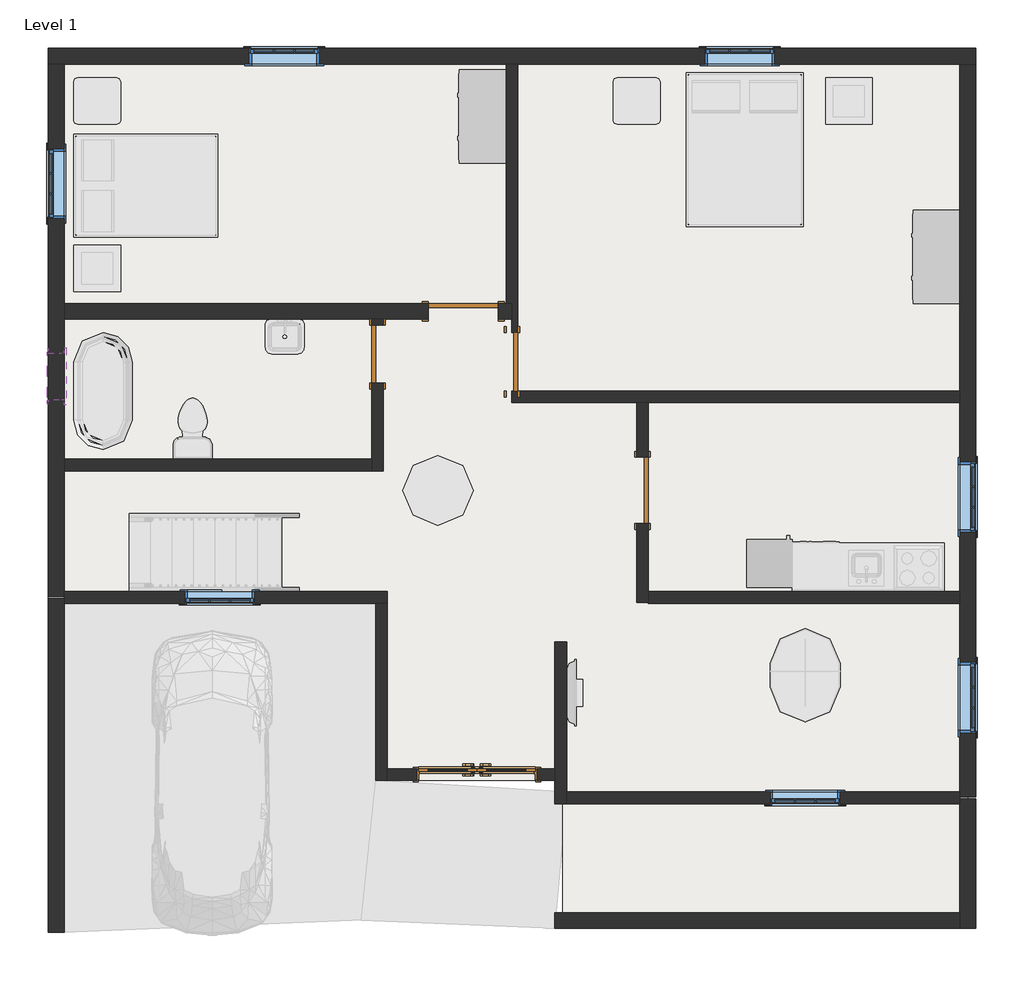
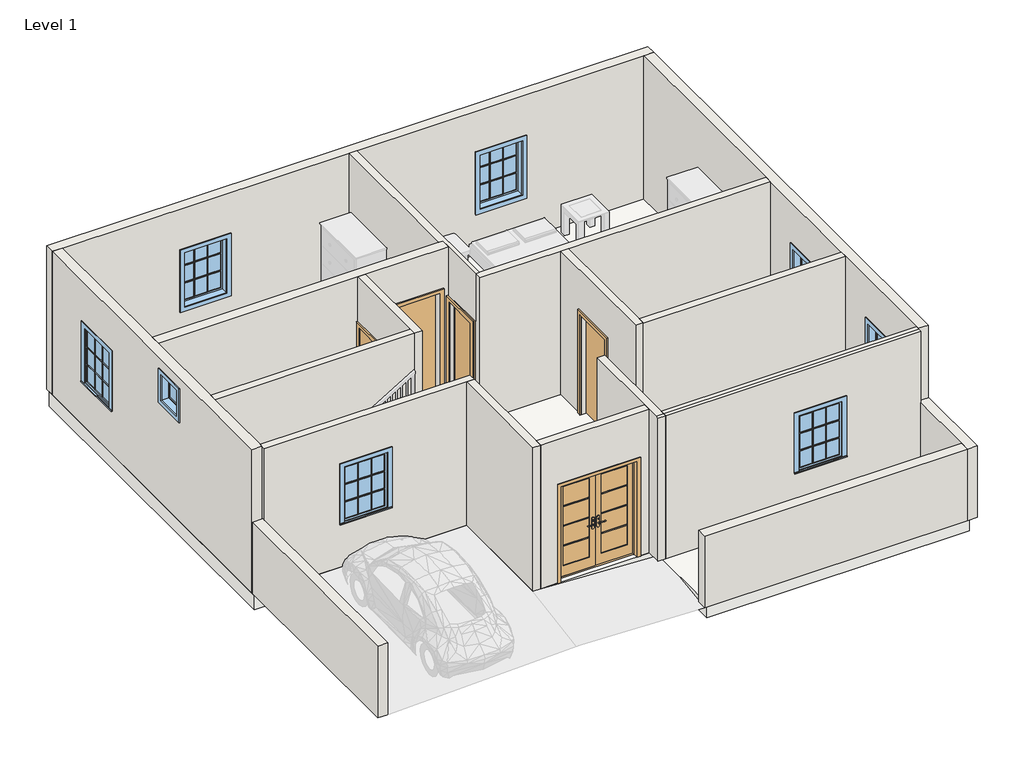
# One storey, part 1 of 2: 18 walls, 8 windows, 5 doors, 1 slab.
"""IFC4 building model written with IfcOpenShell, lengths in millimetres."""

from ifc_helpers import new_model, si_unit, frame, origin, origin_with_axes, place, context, project, spatial, polyline, outline, extrude, faceted_brep, transform, mapped, element, save
from components import door_94998e6c, door_059fdd7e, door_99d96fc5, door_54dd4da4, window_29c06734, window_5c190c7e, window_e41d21a6

model = new_model("IFC4")

# Units and contexts
model_context = context("Model", 3, world=origin())
ifc_project = project(units=[si_unit("LENGTHUNIT", "METRE", prefix="MILLI")], contexts=[model_context])

# Site, building, storey
site = spatial("IfcSite", under=ifc_project)
building = spatial("IfcBuilding", under=site)
storey = spatial("IfcBuildingStorey", under=building, Name="Level 1", Elevation=0.0)

# Doors
placement = place(None, origin())
door_shape = door_94998e6c(model_context)
element("IfcDoor", 1, ObjectType="Door-Exterior-Double-Full Glass-Wood_Clad : 60\" x 80\"", at=placement, inside=storey, context=model_context, shape_type="MappedRepresentation", body=[
    mapped(door_shape, transform((-8502.4576657, 4160.7479822, 0.0), x_axis=(1.0, 0.0, 0.0), y_axis=(0.0, 1.0, 0.0), z_axis=(0.0, 0.0, 1.0))),
])
door_2_shape = door_059fdd7e(model_context)
element("IfcDoor", 2, ObjectType="Single-Flush : 30\" x 80\"", at=placement, inside=storey, context=model_context, shape_type="MappedRepresentation", body=[
    mapped(door_2_shape, transform((-9797.8576657, 9643.9729822, 0.0), x_axis=(0.0, 1.0, 0.0), y_axis=(-1.0, 0.0, 0.0), z_axis=(0.0, 0.0, 1.0))),
])
element("IfcDoor", 3, ObjectType="Single-Flush : 30\" x 80\"", at=placement, inside=storey, context=model_context, shape_type="MappedRepresentation", body=[
    mapped(door_2_shape, transform((-8045.2576657, 9542.3729822, 0.0), x_axis=(0.0, -1.0, 0.0), y_axis=(1.0, 0.0, 0.0), z_axis=(0.0, 0.0, 1.0))),
])
door_3_shape = door_99d96fc5(model_context)
element("IfcDoor", 4, ObjectType="Single-Flush : 34\" x 84\"", at=placement, inside=storey, context=model_context, shape_type="MappedRepresentation", body=[
    mapped(door_3_shape, transform((-6343.4576657, 7865.9729822, 0.0), x_axis=(0.0, 1.0, 0.0), y_axis=(-1.0, 0.0, 0.0), z_axis=(0.0, 0.0, 1.0))),
])
door_4_shape = door_54dd4da4(model_context)
element("IfcDoor", 5, ObjectType="Single-Flush : 36\" x 84\"", at=placement, inside=storey, context=model_context, shape_type="MappedRepresentation", body=[
    mapped(door_4_shape, transform((-8680.2576657, 10202.7729822, 0.0), x_axis=(1.0, 0.0, 0.0), y_axis=(0.0, 1.0, 0.0), z_axis=(0.0, 0.0, 1.0))),
])

# Slab
element("IfcSlab", 6, ObjectType="Generic - 12\"", at=placement, inside=storey, context=model_context, shape_type="SweptSolid", body=[
    extrude(outline(polyline([(-2101.6576657, 13530.1729822), (-2101.6576657, 2252.5729822), (-7384.8576657, 2252.5729822), (-7384.8576657, 4081.3729822), (-9823.2576657, 4081.3729822), (-9823.2576657, 6392.7729822), (-14090.4576657, 6392.7729822), (-14090.4576657, 13530.1729822), (-2101.6576657, 13530.1729822)])), frame((0.0, 0.0, -304.8), z_axis=(0.0, 0.0, 1.0), x_axis=(1.0, 0.0, 0.0)), (0.0, 0.0, 1.0), 304.8),
])

# Walls
element("IfcWall", 7, ObjectType="Generic - 5'", at=placement, inside=storey, context=model_context, shape_type="SweptSolid", body=[
    extrude(outline(polyline([(-7486.4576657, 2354.1729822), (-2203.2576657, 2354.1729822), (-2203.2576657, 2150.9729822), (-7486.4576657, 2150.9729822), (-7486.4576657, 2354.1729822)])), origin_with_axes(), (0.0, 0.0, 1.0), 1524.0),
])
element("IfcWall", 8, ObjectType="Generic - 5'", at=placement, inside=storey, context=model_context, shape_type="SweptSolid", body=[
    extrude(outline(polyline([(-13887.2576657, 6456.2729822), (-13887.2576657, 2100.1729822), (-14090.4576657, 2100.1729822), (-14090.4576657, 6456.2729822), (-13887.2576657, 6456.2729822)])), origin_with_axes(), (0.0, 0.0, 1.0), 1524.0),
])
element("IfcWall", 9, ObjectType="Generic - 5'", at=placement, inside=storey, context=model_context, shape_type="Brep", body=[
    faceted_brep([(-2203.2576657, 3840.0729822, 0.0), (-2203.2576657, 3776.5729822, 0.0), (-2203.2576657, 2354.1729822, 0.0), (-2203.2576657, 2150.9729822, 0.0), (-2203.2576657, 2150.9729822, 1524.0), (-2203.2576657, 2354.1729822, 1524.0), (-2203.2576657, 3840.0729822, 1524.0), (-2000.0576657, 3840.0729822, 0.0), (-2000.0576657, 3840.0729822, 1524.0), (-2000.0576657, 2150.9729822, 1524.0), (-2000.0576657, 2150.9729822, 0.0)], [[[0, 1, 2, 3, 4, 5, 6]], [[7, 8, 9, 10]], [[3, 2, 1, 0, 7, 10]], [[6, 5, 4, 9, 8]], [[0, 6, 8, 7]], [[4, 3, 10, 9]]]),
])
element("IfcWall", 10, ObjectType="Generic - 8\"", at=placement, inside=storey, context=model_context, shape_type="Brep", body=[
    faceted_brep([(-14090.4576657, 13428.5729822, 0.0), (-13887.2576657, 13428.5729822, 0.0), (-8121.4576657, 13428.5729822, 0.0), (-7969.0576657, 13428.5729822, 0.0), (-2203.2576657, 13428.5729822, 0.0), (-2000.0576657, 13428.5729822, 0.0), (-2000.0576657, 13428.5729822, 3048.0), (-2203.2576657, 13428.5729822, 3048.0), (-7969.0576657, 13428.5729822, 3048.0), (-8121.4576657, 13428.5729822, 3048.0), (-13887.2576657, 13428.5729822, 3048.0), (-14090.4576657, 13428.5729822, 3048.0), (-10559.8576657, 13428.5729822, 2133.6), (-10559.8576657, 13428.5729822, 914.4), (-11474.2576657, 13428.5729822, 914.4), (-11474.2576657, 13428.5729822, 2133.6), (-4616.2576657, 13428.5729822, 2133.6), (-4616.2576657, 13428.5729822, 914.4), (-5530.6576657, 13428.5729822, 914.4), (-5530.6576657, 13428.5729822, 2133.6), (-14090.4576657, 13631.7729822, 0.0), (-14090.4576657, 13631.7729822, 3048.0), (-2000.0576657, 13631.7729822, 3048.0), (-2000.0576657, 13631.7729822, 0.0), (-10559.8576657, 13631.7729822, 2133.6), (-11474.2576657, 13631.7729822, 2133.6), (-11474.2576657, 13631.7729822, 914.4), (-10559.8576657, 13631.7729822, 914.4), (-4616.2576657, 13631.7729822, 2133.6), (-5530.6576657, 13631.7729822, 2133.6), (-5530.6576657, 13631.7729822, 914.4), (-4616.2576657, 13631.7729822, 914.4)], [[[0, 1, 2, 3, 4, 5, 6, 7, 8, 9, 10, 11], [12, 13, 14, 15], [16, 17, 18, 19]], [[20, 21, 22, 23], [24, 25, 26, 27], [28, 29, 30, 31]], [[5, 4, 3, 2, 1, 0, 20, 23]], [[6, 5, 23, 22]], [[0, 11, 21, 20]], [[13, 12, 24, 27]], [[14, 13, 27, 26]], [[15, 14, 26, 25]], [[12, 15, 25, 24]], [[17, 16, 28, 31]], [[18, 17, 31, 30]], [[19, 18, 30, 29]], [[16, 19, 29, 28]], [[11, 10, 9, 8, 7, 6, 22, 21]]]),
])
element("IfcWall", 11, ObjectType="Generic - 8\"", at=placement, inside=storey, context=model_context, shape_type="Brep", body=[
    faceted_brep([(-2203.2576657, 13428.5729822, 0.0), (-2203.2576657, 9161.3729822, 0.0), (-2203.2576657, 9008.9729822, 0.0), (-2203.2576657, 6545.1729822, 0.0), (-2203.2576657, 6392.7729822, 0.0), (-2203.2576657, 3865.4729822, 0.0), (-2203.2576657, 3865.4729822, 3048.0), (-2203.2576657, 6392.7729822, 3048.0), (-2203.2576657, 6545.1729822, 3048.0), (-2203.2576657, 9008.9729822, 3048.0), (-2203.2576657, 9161.3729822, 3048.0), (-2203.2576657, 13428.5729822, 3048.0), (-2203.2576657, 7319.8729822, 2133.6), (-2203.2576657, 7319.8729822, 914.4), (-2203.2576657, 8234.2729822, 914.4), (-2203.2576657, 8234.2729822, 2133.6), (-2203.2576657, 4703.6729822, 2133.6), (-2203.2576657, 4703.6729822, 914.4), (-2203.2576657, 5618.0729822, 914.4), (-2203.2576657, 5618.0729822, 2133.6), (-2000.0576657, 13428.5729822, 0.0), (-2000.0576657, 13428.5729822, 3048.0), (-2000.0576657, 3865.4729822, 3048.0), (-2000.0576657, 3865.4729822, 0.0), (-2000.0576657, 7319.8729822, 2133.6), (-2000.0576657, 8234.2729822, 2133.6), (-2000.0576657, 8234.2729822, 914.4), (-2000.0576657, 7319.8729822, 914.4), (-2000.0576657, 4703.6729822, 2133.6), (-2000.0576657, 5618.0729822, 2133.6), (-2000.0576657, 5618.0729822, 914.4), (-2000.0576657, 4703.6729822, 914.4)], [[[0, 1, 2, 3, 4, 5, 6, 7, 8, 9, 10, 11], [12, 13, 14, 15], [16, 17, 18, 19]], [[20, 21, 22, 23], [24, 25, 26, 27], [28, 29, 30, 31]], [[5, 4, 3, 2, 1, 0, 20, 23]], [[6, 5, 23, 22]], [[0, 11, 21, 20]], [[13, 12, 24, 27]], [[14, 13, 27, 26]], [[15, 14, 26, 25]], [[12, 15, 25, 24]], [[17, 16, 28, 31]], [[18, 17, 31, 30]], [[19, 18, 30, 29]], [[16, 19, 29, 28]], [[11, 10, 9, 8, 7, 6, 22, 21]]]),
])
element("IfcWall", 12, ObjectType="Generic - 8\"", at=placement, inside=storey, context=model_context, shape_type="Brep", body=[
    faceted_brep([(-8045.2576657, 10304.3729822, 0.0), (-8121.4576657, 10304.3729822, 0.0), (-8223.0576657, 10304.3729822, 0.0), (-8223.0576657, 10304.3729822, 2133.6), (-9137.4576657, 10304.3729822, 2133.6), (-9137.4576657, 10304.3729822, 0.0), (-13887.2576657, 10304.3729822, 0.0), (-13887.2576657, 10304.3729822, 3048.0), (-8121.4576657, 10304.3729822, 3048.0), (-8045.2576657, 10304.3729822, 3048.0), (-8223.0576657, 10101.1729822, 2133.6), (-8223.0576657, 10101.1729822, 0.0), (-8045.2576657, 10101.1729822, 0.0), (-8045.2576657, 10101.1729822, 3048.0), (-9721.6576657, 10101.1729822, 3048.0), (-9874.0576657, 10101.1729822, 3048.0), (-13887.2576657, 10101.1729822, 3048.0), (-13887.2576657, 10101.1729822, 0.0), (-9874.0576657, 10101.1729822, 0.0), (-9721.6576657, 10101.1729822, 0.0), (-9137.4576657, 10101.1729822, 0.0), (-9137.4576657, 10101.1729822, 2133.6)], [[[0, 1, 2, 3, 4, 5, 6, 7, 8, 9]], [[10, 11, 12, 13, 14, 15, 16, 17, 18, 19, 20, 21]], [[12, 11, 2, 1, 0]], [[20, 19, 18, 17, 6, 5]], [[0, 9, 13, 12]], [[7, 6, 17, 16]], [[3, 2, 11, 10]], [[4, 3, 10, 21]], [[5, 4, 21, 20]], [[9, 8, 7, 16, 15, 14, 13]]]),
])
element("IfcWall", 13, ObjectType="Generic - 8\"", at=placement, inside=storey, context=model_context, shape_type="Brep", body=[
    faceted_brep([(-13887.2576657, 6481.6729822, 0.0), (-13887.2576657, 6545.1729822, 0.0), (-13887.2576657, 8119.9729822, 0.0), (-13887.2576657, 8272.3729822, 0.0), (-13887.2576657, 10101.1729822, 0.0), (-13887.2576657, 10304.3729822, 0.0), (-13887.2576657, 13428.5729822, 0.0), (-13887.2576657, 13428.5729822, 3048.0), (-13887.2576657, 10304.3729822, 3048.0), (-13887.2576657, 10101.1729822, 3048.0), (-13887.2576657, 8272.3729822, 3048.0), (-13887.2576657, 8119.9729822, 3048.0), (-13887.2576657, 6545.1729822, 3048.0), (-13887.2576657, 6481.6729822, 3048.0), (-13887.2576657, 12323.6729822, 2133.6), (-13887.2576657, 12323.6729822, 914.4), (-13887.2576657, 11409.2729822, 914.4), (-13887.2576657, 11409.2729822, 2133.6), (-13887.2576657, 9047.0729822, 2768.6), (-13887.2576657, 9656.6729822, 2768.6), (-13887.2576657, 9656.6729822, 2159.0), (-13887.2576657, 9047.0729822, 2159.0), (-14090.4576657, 6481.6729822, 0.0), (-14090.4576657, 6481.6729822, 3048.0), (-14090.4576657, 13428.5729822, 3048.0), (-14090.4576657, 13428.5729822, 0.0), (-14090.4576657, 12323.6729822, 2133.6), (-14090.4576657, 11409.2729822, 2133.6), (-14090.4576657, 11409.2729822, 914.4), (-14090.4576657, 12323.6729822, 914.4), (-14090.4576657, 9047.0729822, 2768.6), (-14090.4576657, 9047.0729822, 2159.0), (-14090.4576657, 9656.6729822, 2159.0), (-14090.4576657, 9656.6729822, 2768.6)], [[[0, 1, 2, 3, 4, 5, 6, 7, 8, 9, 10, 11, 12, 13], [14, 15, 16, 17], [18, 19, 20, 21]], [[22, 23, 24, 25], [26, 27, 28, 29], [30, 31, 32, 33]], [[6, 5, 4, 3, 2, 1, 0, 22, 25]], [[0, 13, 23, 22]], [[7, 6, 25, 24]], [[14, 17, 27, 26]], [[17, 16, 28, 27]], [[16, 15, 29, 28]], [[15, 14, 26, 29]], [[30, 33, 19, 18]], [[33, 32, 20, 19]], [[32, 31, 21, 20]], [[31, 30, 18, 21]], [[13, 12, 11, 10, 9, 8, 7, 24, 23]]]),
])
element("IfcWall", 14, ObjectType="INNER 6\"", at=placement, inside=storey, context=model_context, shape_type="Brep", body=[
    faceted_brep([(-8121.4576657, 13428.5729822, 0.0), (-8121.4576657, 10304.3729822, 0.0), (-8121.4576657, 10304.3729822, 3048.0), (-8121.4576657, 13428.5729822, 3048.0), (-7969.0576657, 13428.5729822, 0.0), (-7969.0576657, 13428.5729822, 3048.0), (-7969.0576657, 9161.3729822, 3048.0), (-7969.0576657, 9161.3729822, 2032.0), (-7969.0576657, 9923.3729822, 2032.0), (-7969.0576657, 9923.3729822, 0.0), (-8045.2576657, 9923.3729822, 0.0), (-8045.2576657, 10101.1729822, 0.0), (-8045.2576657, 10304.3729822, 0.0), (-8045.2576657, 10304.3729822, 3048.0), (-8045.2576657, 9923.3729822, 2032.0), (-8045.2576657, 9161.3729822, 2032.0), (-8045.2576657, 9161.3729822, 3048.0), (-8045.2576657, 10101.1729822, 3048.0)], [[[0, 1, 2, 3]], [[4, 5, 6, 7, 8, 9]], [[1, 0, 4, 9, 10, 11, 12]], [[0, 3, 5, 4]], [[2, 1, 12, 13]], [[13, 12, 11, 10, 14, 15, 16, 17]], [[6, 16, 15, 7]], [[14, 8, 7, 15]], [[8, 14, 10, 9]], [[3, 2, 13, 17, 16, 6, 5]]]),
])
element("IfcWall", 15, ObjectType="INNER 6\"", at=placement, inside=storey, context=model_context, shape_type="Brep", body=[
    faceted_brep([(-2203.2576657, 9161.3729822, 0.0), (-8045.2576657, 9161.3729822, 0.0), (-8045.2576657, 9161.3729822, 2032.0), (-8045.2576657, 9161.3729822, 3048.0), (-7969.0576657, 9161.3729822, 3048.0), (-2203.2576657, 9161.3729822, 3048.0), (-2203.2576657, 9008.9729822, 0.0), (-2203.2576657, 9008.9729822, 3048.0), (-6267.2576657, 9008.9729822, 3048.0), (-6419.6576657, 9008.9729822, 3048.0), (-8045.2576657, 9008.9729822, 3048.0), (-8045.2576657, 9008.9729822, 0.0), (-6419.6576657, 9008.9729822, 0.0), (-6267.2576657, 9008.9729822, 0.0)], [[[0, 1, 2, 3, 4, 5]], [[6, 7, 8, 9, 10, 11, 12, 13]], [[1, 0, 6, 13, 12, 11]], [[3, 2, 1, 11, 10]], [[0, 5, 7, 6]], [[5, 4, 3, 10, 9, 8, 7]]]),
])
element("IfcWall", 16, ObjectType="INNER 6\"", at=placement, inside=storey, context=model_context, shape_type="Brep", body=[
    faceted_brep([(-9874.0576657, 10101.1729822, 0.0), (-9874.0576657, 10024.9729822, 0.0), (-9874.0576657, 10024.9729822, 2032.0), (-9874.0576657, 9262.9729822, 2032.0), (-9874.0576657, 9262.9729822, 0.0), (-9874.0576657, 8272.3729822, 0.0), (-9874.0576657, 8119.9729822, 0.0), (-9874.0576657, 8119.9729822, 3048.0), (-9874.0576657, 8272.3729822, 3048.0), (-9874.0576657, 10101.1729822, 3048.0), (-9721.6576657, 10024.9729822, 2032.0), (-9721.6576657, 10024.9729822, 0.0), (-9721.6576657, 10101.1729822, 0.0), (-9721.6576657, 10101.1729822, 3048.0), (-9721.6576657, 8119.9729822, 3048.0), (-9721.6576657, 8119.9729822, 0.0), (-9721.6576657, 9262.9729822, 0.0), (-9721.6576657, 9262.9729822, 2032.0)], [[[0, 1, 2, 3, 4, 5, 6, 7, 8, 9]], [[10, 11, 12, 13, 14, 15, 16, 17]], [[16, 15, 6, 5, 4]], [[12, 11, 1, 0]], [[0, 9, 13, 12]], [[7, 6, 15, 14]], [[2, 1, 11, 10]], [[3, 2, 10, 17]], [[4, 3, 17, 16]], [[9, 8, 7, 14, 13]]]),
])
element("IfcWall", 17, ObjectType="INNER 6\"", at=placement, inside=storey, context=model_context, shape_type="SweptSolid", body=[
    extrude(outline(polyline([(-13887.2576657, 8272.3729822), (-9874.0576657, 8272.3729822), (-9874.0576657, 8119.9729822), (-13887.2576657, 8119.9729822), (-13887.2576657, 8272.3729822)])), origin_with_axes(), (0.0, 0.0, 1.0), 3048.0),
])
element("IfcWall", 18, ObjectType="INNER 6\"", at=placement, inside=storey, context=model_context, shape_type="Brep", body=[
    faceted_brep([(-13887.2576657, 6392.7729822, 0.0), (-9823.2576657, 6392.7729822, 0.0), (-9670.8576657, 6392.7729822, 0.0), (-9670.8576657, 6392.7729822, 3048.0), (-9823.2576657, 6392.7729822, 3048.0), (-13887.2576657, 6392.7729822, 3048.0), (-12312.4576657, 6392.7729822, 2133.6), (-11398.0576657, 6392.7729822, 2133.6), (-11398.0576657, 6392.7729822, 914.4), (-12312.4576657, 6392.7729822, 914.4), (-13887.2576657, 6545.1729822, 0.0), (-13887.2576657, 6545.1729822, 3048.0), (-9670.8576657, 6545.1729822, 3048.0), (-9670.8576657, 6545.1729822, 0.0), (-12312.4576657, 6545.1729822, 2133.6), (-12312.4576657, 6545.1729822, 914.4), (-11398.0576657, 6545.1729822, 914.4), (-11398.0576657, 6545.1729822, 2133.6), (-13887.2576657, 6481.6729822, 0.0), (-13887.2576657, 6481.6729822, 3048.0)], [[[0, 1, 2, 3, 4, 5], [6, 7, 8, 9]], [[10, 11, 12, 13], [14, 15, 16, 17]], [[2, 1, 0, 18, 10, 13]], [[0, 5, 19, 11, 10, 18]], [[3, 2, 13, 12]], [[15, 14, 6, 9]], [[16, 15, 9, 8]], [[17, 16, 8, 7]], [[14, 17, 7, 6]], [[5, 4, 3, 12, 11, 19]]]),
])
element("IfcWall", 19, ObjectType="INNER 6\"", at=placement, inside=storey, context=model_context, shape_type="Brep", body=[
    faceted_brep([(-6419.6576657, 9008.9729822, 0.0), (-6419.6576657, 8297.7729822, 0.0), (-6419.6576657, 8297.7729822, 2133.6), (-6419.6576657, 7434.1729822, 2133.6), (-6419.6576657, 7434.1729822, 0.0), (-6419.6576657, 6405.4729822, 0.0), (-6419.6576657, 6405.4729822, 3048.0), (-6419.6576657, 9008.9729822, 3048.0), (-6267.2576657, 8297.7729822, 2133.6), (-6267.2576657, 8297.7729822, 0.0), (-6267.2576657, 9008.9729822, 0.0), (-6267.2576657, 9008.9729822, 3048.0), (-6267.2576657, 6545.1729822, 3048.0), (-6267.2576657, 6405.4729822, 3048.0), (-6267.2576657, 6405.4729822, 0.0), (-6267.2576657, 6545.1729822, 0.0), (-6267.2576657, 7434.1729822, 0.0), (-6267.2576657, 7434.1729822, 2133.6)], [[[0, 1, 2, 3, 4, 5, 6, 7]], [[8, 9, 10, 11, 12, 13, 14, 15, 16, 17]], [[10, 9, 1, 0]], [[16, 15, 14, 5, 4]], [[6, 5, 14, 13]], [[0, 7, 11, 10]], [[2, 1, 9, 8]], [[3, 2, 8, 17]], [[4, 3, 17, 16]], [[7, 6, 13, 12, 11]]]),
])
element("IfcWall", 20, ObjectType="INNER 6\"", at=placement, inside=storey, context=model_context, shape_type="Brep", body=[
    faceted_brep([(-6267.2576657, 6392.7729822, 0.0), (-2203.2576657, 6392.7729822, 0.0), (-2203.2576657, 6392.7729822, 3048.0), (-6267.2576657, 6392.7729822, 3048.0), (-6267.2576657, 6545.1729822, 0.0), (-6267.2576657, 6545.1729822, 3048.0), (-2203.2576657, 6545.1729822, 3048.0), (-2203.2576657, 6545.1729822, 0.0), (-6267.2576657, 6405.4729822, 0.0), (-6267.2576657, 6405.4729822, 3048.0)], [[[0, 1, 2, 3]], [[4, 5, 6, 7]], [[1, 0, 8, 4, 7]], [[2, 1, 7, 6]], [[0, 3, 9, 5, 4, 8]], [[3, 2, 6, 5, 9]]]),
])
element("IfcWall", 21, ObjectType="INNER 6\"", at=placement, inside=storey, context=model_context, shape_type="Brep", body=[
    faceted_brep([(-7334.0576657, 3776.5729822, 0.0), (-2203.2576657, 3776.5729822, 0.0), (-2203.2576657, 3776.5729822, 3048.0), (-7334.0576657, 3776.5729822, 3048.0), (-4679.7576657, 3776.5729822, 2133.6), (-3765.3576657, 3776.5729822, 2133.6), (-3765.3576657, 3776.5729822, 914.4), (-4679.7576657, 3776.5729822, 914.4), (-7334.0576657, 3928.9729822, 0.0), (-7334.0576657, 3928.9729822, 3048.0), (-2203.2576657, 3928.9729822, 3048.0), (-2203.2576657, 3928.9729822, 0.0), (-4679.7576657, 3928.9729822, 2133.6), (-4679.7576657, 3928.9729822, 914.4), (-3765.3576657, 3928.9729822, 914.4), (-3765.3576657, 3928.9729822, 2133.6), (-2203.2576657, 3840.0729822, 0.0), (-2203.2576657, 3840.0729822, 3048.0), (-7334.0576657, 3840.0729822, 3048.0)], [[[0, 1, 2, 3], [4, 5, 6, 7]], [[8, 9, 10, 11], [12, 13, 14, 15]], [[1, 0, 8, 11, 16]], [[2, 1, 16, 11, 10, 17]], [[0, 3, 18, 9, 8]], [[13, 12, 4, 7]], [[14, 13, 7, 6]], [[15, 14, 6, 5]], [[12, 15, 5, 4]], [[3, 2, 17, 18]], [[17, 10, 9, 18]]]),
])
element("IfcWall", 22, ObjectType="INNER 6\"", at=placement, inside=storey, context=model_context, shape_type="Brep", body=[
    faceted_brep([(-9823.2576657, 6392.7729822, 0.0), (-9823.2576657, 4081.3729822, 0.0), (-9823.2576657, 4081.3729822, 3048.0), (-9823.2576657, 6392.7729822, 3048.0), (-9670.8576657, 6392.7729822, 0.0), (-9670.8576657, 6392.7729822, 3048.0), (-9670.8576657, 4233.7729822, 3048.0), (-9670.8576657, 4081.3729822, 3048.0), (-9670.8576657, 4081.3729822, 0.0), (-9670.8576657, 4233.7729822, 0.0)], [[[0, 1, 2, 3]], [[4, 5, 6, 7, 8, 9]], [[1, 0, 4, 9, 8]], [[2, 1, 8, 7]], [[0, 3, 5, 4]], [[3, 2, 7, 6, 5]]]),
])
element("IfcWall", 23, ObjectType="INNER 6\"", at=placement, inside=storey, context=model_context, shape_type="SweptSolid", body=[
    extrude(outline(polyline([(0.0, -7486.4576657), (3048.0, -7486.4576657), (3048.0, -9670.8576657), (0.0, -9670.8576657), (0.0, -9289.8576657), (2057.4, -9289.8576657), (2057.4, -7715.0576657), (0.0, -7715.0576657), (0.0, -7486.4576657)])), frame((0.0, 4081.3729822, 0.0), z_axis=(0.0, 1.0, 0.0), x_axis=(0.0, 0.0, 1.0)), (0.0, 0.0, 1.0), 152.4),
])
element("IfcWall", 24, ObjectType="INNER 6\"", at=placement, inside=storey, context=model_context, shape_type="Brep", body=[
    faceted_brep([(-7486.4576657, 5884.7729822, 0.0), (-7486.4576657, 4233.7729822, 0.0), (-7486.4576657, 4081.3729822, 0.0), (-7486.4576657, 3776.5729822, 0.0), (-7486.4576657, 3776.5729822, 3048.0), (-7486.4576657, 3840.0729822, 3048.0), (-7486.4576657, 4081.3729822, 3048.0), (-7486.4576657, 4233.7729822, 3048.0), (-7486.4576657, 5884.7729822, 3048.0), (-7334.0576657, 5884.7729822, 0.0), (-7334.0576657, 5884.7729822, 3048.0), (-7334.0576657, 3928.9729822, 3048.0), (-7334.0576657, 3840.0729822, 3048.0), (-7334.0576657, 3776.5729822, 3048.0), (-7334.0576657, 3776.5729822, 0.0), (-7334.0576657, 3928.9729822, 0.0)], [[[0, 1, 2, 3, 4, 5, 6, 7, 8]], [[9, 10, 11, 12, 13, 14, 15]], [[3, 2, 1, 0, 9, 15, 14]], [[0, 8, 10, 9]], [[4, 3, 14, 13]], [[5, 4, 13, 12]], [[8, 7, 6, 5, 12, 11, 10]]]),
])

# Windows
window_shape = window_29c06734(model_context)
element("IfcWindow", 25, ObjectType="Casement 3x3 with Trim : 36\" x 48\"", at=placement, inside=storey, context=model_context, shape_type="MappedRepresentation", body=[
    mapped(window_shape, transform((-11017.0576657, 13530.1729822, 0.0), x_axis=(1.0, 0.0, 0.0), y_axis=(0.0, 1.0, 0.0), z_axis=(0.0, 0.0, 1.0))),
])
element("IfcWindow", 26, ObjectType="Casement 3x3 with Trim : 36\" x 48\"", at=placement, inside=storey, context=model_context, shape_type="MappedRepresentation", body=[
    mapped(window_shape, transform((-5073.4576657, 13530.1729822, 0.0), x_axis=(1.0, 0.0, 0.0), y_axis=(0.0, 1.0, 0.0), z_axis=(0.0, 0.0, 1.0))),
])
element("IfcWindow", 27, ObjectType="Casement 3x3 with Trim : 36\" x 48\"", at=placement, inside=storey, context=model_context, shape_type="MappedRepresentation", body=[
    mapped(window_shape, transform((-2101.6576657, 7777.0729822, 0.0), x_axis=(0.0, -1.0, 0.0), y_axis=(1.0, 0.0, 0.0), z_axis=(0.0, 0.0, 1.0))),
])
element("IfcWindow", 28, ObjectType="Casement 3x3 with Trim : 36\" x 48\"", at=placement, inside=storey, context=model_context, shape_type="MappedRepresentation", body=[
    mapped(window_shape, transform((-2101.6576657, 5160.8729822, 0.0), x_axis=(0.0, -1.0, 0.0), y_axis=(1.0, 0.0, 0.0), z_axis=(0.0, 0.0, 1.0))),
])
element("IfcWindow", 29, ObjectType="Casement 3x3 with Trim : 36\" x 48\"", at=placement, inside=storey, context=model_context, shape_type="MappedRepresentation", body=[
    mapped(window_shape, transform((-13988.8576657, 11866.4729822, 0.0), x_axis=(0.0, 1.0, 0.0), y_axis=(-1.0, 0.0, 0.0), z_axis=(0.0, 0.0, 1.0))),
])
window_2_shape = window_5c190c7e(model_context)
element("IfcWindow", 30, ObjectType="Casement 3x3 with Trim : 36\" x 48\"", at=placement, inside=storey, context=model_context, shape_type="MappedRepresentation", body=[
    mapped(window_2_shape, transform((-4222.5576657, 3852.7729822, 0.0), x_axis=(-1.0, 0.0, 0.0), y_axis=(0.0, -1.0, 0.0), z_axis=(0.0, 0.0, 1.0))),
])
element("IfcWindow", 31, ObjectType="Casement 3x3 with Trim : 36\" x 48\"", at=placement, inside=storey, context=model_context, shape_type="MappedRepresentation", body=[
    mapped(window_2_shape, transform((-11855.2576657, 6468.9729822, 0.0), x_axis=(-1.0, 0.0, 0.0), y_axis=(0.0, -1.0, 0.0), z_axis=(0.0, 0.0, 1.0))),
])
window_3_shape = window_e41d21a6(model_context)
element("IfcWindow", 32, ObjectType="Transom with Trim : 24\" x 24\"", at=placement, inside=storey, context=model_context, shape_type="MappedRepresentation", body=[
    mapped(window_3_shape, transform((-13988.8576657, 9313.7729822, 0.0), x_axis=(0.0, -1.0, 0.0), y_axis=(1.0, 0.0, 0.0), z_axis=(0.0, 0.0, 1.0))),
])

save(model, "model.ifc")

# Revit data of these elements
# Type "Door-Exterior-Double-Full Glass-Wood_Clad : 60\" x 80\""
#   Type Mark = "9"
#   Assembly Code = "B2030100"
#   Analytic Construction = "French door, wood frame with double glass"
#   Top Rail = 0' - 4 11/16"
#   Threshold Offset [instance default] = 0' - 0 1/2"
#   Thickness = 0' - 1 3/8"
#   Thermal Resistance (R) = 1.9158 (h·ft²·°F)/BTU
#   Swing Angle [instance default] = 90.00°
#   Stiles = 0' - 4 3/4"
#   Rough Width = 5' - 2"
#   Rough Height = 6' - 9"
#   Panel Width = 2' - 6"
#   Door Offset [instance default] = 0' - 0"
#   Height = 6' - 8"
#   Width = 5' - 0"
#   Heat Transfer Coefficient (U) = 0.5220 BTU/(h·ft²·°F)
#   Bottom Rail = 0' - 9 1/8"
#   Exterior Trim [instance default] = yes
#   Threshold [instance default] = yes
#   Show Grill [instance default] = yes
#   Function = 1
#   Trim Material = Cherry
#   Threshold Material = Cherry
#   Panel Material = Cherry
#   Glazing = Glass
#   Frame Material = Cherry
#   Door Handle Material = Aluminum
#   Visual Light Transmittance = 0
#   Solar Heat Gain Coefficient = 0
#   Wall Closure = (empty or 0)
#   Construction Type = (empty or 0)
# Type "Single-Flush : 30\" x 80\""
#   Type Mark = "5"
#   Construction Type Id = "MDOOR"
#   Assembly Code = "C1020"
#   Analytic Construction = "Metal"
#   Thickness = 0' - 2"
#   Heat Transfer Coefficient (U) = 0.651978 BTU/(h·ft²·°F)
#   Height = 6' - 8"
#   Trim Projection Ext = 0' - 1"
#   Trim Projection Int = 0' - 1"
#   Trim Width = 0' - 3"
#   Width = 2' - 6"
#   Define Thermal Properties by = 1
#   Door Material = Door - Panel
#   Frame Material = Door - Frame
#   Visual Light Transmittance = 0
#   Solar Heat Gain Coefficient = 0
#   Function = (empty or 0)
#   Wall Closure = (empty or 0)
# Type "Single-Flush : 34\" x 84\""
#   Type Mark = "2"
#   Construction Type Id = "MDOOR"
#   Assembly Code = "C1020"
#   Analytic Construction = "Metal"
#   Thickness = 0' - 2"
#   Heat Transfer Coefficient (U) = 0.651978 BTU/(h·ft²·°F)
#   Height = 7' - 0"
#   Trim Projection Ext = 0' - 1"
#   Trim Projection Int = 0' - 1"
#   Trim Width = 0' - 3"
#   Width = 2' - 10"
#   Define Thermal Properties by = 1
#   Door Material = Door - Panel
#   Frame Material = Door - Frame
#   Visual Light Transmittance = 0
#   Solar Heat Gain Coefficient = 0
#   Function = (empty or 0)
#   Wall Closure = (empty or 0)
# Type "Single-Flush : 36\" x 84\""
#   Type Mark = "1"
#   Construction Type Id = "MDOOR"
#   Assembly Code = "C1020"
#   Analytic Construction = "Metal"
#   Thickness = 0' - 2"
#   Heat Transfer Coefficient (U) = 0.651978 BTU/(h·ft²·°F)
#   Height = 7' - 0"
#   Trim Projection Ext = 0' - 1"
#   Trim Projection Int = 0' - 1"
#   Trim Width = 0' - 3"
#   Width = 3' - 0"
#   Define Thermal Properties by = 1
#   Door Material = Door - Panel
#   Frame Material = Door - Frame
#   Visual Light Transmittance = 0
#   Solar Heat Gain Coefficient = 0
#   Function = (empty or 0)
#   Wall Closure = (empty or 0)
# Type "Generic - 12\""
#   Assembly Code = "B1010"
#   Function = 0
#   Layers, outside or top first: 1' - 0" no material (function 1)
# Type "Generic - 5'"
#   Assembly Code = "B2010"
#   Layers, outside or top first: 0' - 8" "Birch" (function 1)
# Type "Generic - 8\""
#   Assembly Code = "B2010"
#   Layers, outside or top first: 0' - 8" "Brick, Common" (function 1)
# Type "INNER 6\""
#   Assembly Code = "B2010"
#   Layers, outside or top first: 0' - 6" "Brick, Common" (function 1)
# Type "Casement 3x3 with Trim : 36\" x 48\""
#   Type Mark = "10"
#   Construction Type Id = "GSP4R"
#   Assembly Code = "B2020100"
#   Analytic Construction = "1/8 in Pilkington single glazing"
#   Visual Light Transmittance = 0.9
#   Solar Heat Gain Coefficient = 0.78
#   Heat Transfer Coefficient (U) = 0.6496 BTU/(h·ft²·°F)
#   Height = 4' - 0"
#   Default Sill Height = 3' - 0"
#   Trim Projection - Ext. = 0' - 0 1/2"
#   Trim Projection - Int. = 0' - 0 3/4"
#   Trim Width - Exterior = 0' - 3 1/2"
#   Trim Width - Interior = 0' - 3 1/2"
#   Width = 3' - 0"
#   Window Inset = 0' - 0 3/4"
#   Define Thermal Properties by = 1
#   Glass Pane Material = Glass
#   Sash Material = Sash
#   Trim Exterior Material = Trim
#   Trim Interior Material = Trim
#   Wall Closure = (empty or 0)
# Type "Transom with Trim : 24\" x 24\""
#   Type Mark = "13"
#   Construction Type Id = "GSP4R"
#   Assembly Code = "B2020100"
#   Analytic Construction = "1/8 in Pilkington single glazing"
#   Visual Light Transmittance = 0.9
#   Solar Heat Gain Coefficient = 0.78
#   Heat Transfer Coefficient (U) = 0.6496 BTU/(h·ft²·°F)
#   Height = 2' - 0"
#   Default Sill Height = 7' - 1"
#   Trim Projection - Ext. = 0' - 0 1/2"
#   Trim Projection - Int. = 0' - 0 3/4"
#   Trim Width - Exterior = 0' - 3 1/2"
#   Trim Width - Interior = 0' - 3 1/2"
#   Width = 2' - 0"
#   Window Inset = 0' - 0 3/4"
#   Define Thermal Properties by = 1
#   Glass Pane Material = Glass
#   Sash Material = Sash
#   Trim Exterior Material = Trim
#   Trim Interior Material = Trim
#   Wall Closure = (empty or 0)
# Element 1 (IfcDoor, "Door-Exterior-Double-Full Glass-Wood_Clad : 60\" x 80\"")
#   Threshold Offset = 0' - 0 1/2"
#   Swing Angle = 90.00°
#   Door Offset = 0' - 0"
#   Threshold = yes
#   Show Grill = yes
#   Exterior Trim = yes
#   Phase Created = New Construction
#   Materials on its faces: "Cherry", "Aluminum", "Glass"
# Elements 2, 3 (IfcDoor, "Single-Flush : 30\" x 80\"")
#   Phase Created = New Construction
#   Materials on its faces: "Door - Frame", "Door - Panel"
# Element 4 (IfcDoor, "Single-Flush : 34\" x 84\"")
#   Phase Created = New Construction
#   Materials on its faces: "Door - Frame", "Door - Panel"
# Element 5 (IfcDoor, "Single-Flush : 36\" x 84\"")
#   Phase Created = New Construction
#   Materials on its faces: "Door - Frame", "Door - Panel"
# Element 6 (IfcSlab, "Generic - 12\"")
#   Height Offset From Level = 0' - 0"
#   Phase Created = New Construction
#   Materials on its faces: "Default Floor"
# Elements 7, 8, 9 (IfcWall, "Generic - 5'")
#   Top Offset = 0' - 0"
#   Base Offset = 0' - 0"
#   Unconnected Height = 5' - 0"
#   wall height = 5' - 0"
#   Phase Created = New Construction
#   Base Constraint = Level 1
#   Materials on its faces: "Birch"
# Elements 10, 11, 12, 13 (IfcWall, "Generic - 8\"")
#   Top Offset = 0' - 0"
#   Base Offset = 0' - 0"
#   Unconnected Height = 10' - 0"
#   wall height = 10' - 0"
#   Phase Created = New Construction
#   Base Constraint = Level 1
#   Materials on its faces: "Brick, Common"
# Elements 14, 15, 16, 17, 18, 19, 20, 21, 22, 23, 24 (IfcWall, "INNER 6\"")
#   Top Offset = 0' - 0"
#   Base Offset = 0' - 0"
#   Unconnected Height = 10' - 0"
#   wall height = 10' - 0"
#   Phase Created = New Construction
#   Base Constraint = Level 1
#   Materials on its faces: "Brick, Common"
# Element 25 (IfcWindow, "Casement 3x3 with Trim : 36\" x 48\"")
#   Mark = "1"
#   Phase Created = New Construction
#   Materials on its faces: "Sash", "Glass", "Trim"
# Element 26 (IfcWindow, "Casement 3x3 with Trim : 36\" x 48\"")
#   Mark = "2"
#   Phase Created = New Construction
#   Materials on its faces: "Sash", "Glass", "Trim"
# Element 27 (IfcWindow, "Casement 3x3 with Trim : 36\" x 48\"")
#   Mark = "3"
#   Phase Created = New Construction
#   Materials on its faces: "Sash", "Glass", "Trim"
# Element 28 (IfcWindow, "Casement 3x3 with Trim : 36\" x 48\"")
#   Mark = "4"
#   Phase Created = New Construction
#   Materials on its faces: "Sash", "Glass", "Trim"
# Element 29 (IfcWindow, "Casement 3x3 with Trim : 36\" x 48\"")
#   Mark = "7"
#   Phase Created = New Construction
#   Materials on its faces: "Sash", "Glass", "Trim"
# Element 30 (IfcWindow, "Casement 3x3 with Trim : 36\" x 48\"")
#   Mark = "5"
#   Phase Created = New Construction
#   Materials on its faces: "Sash", "Glass", "Trim"
# Element 31 (IfcWindow, "Casement 3x3 with Trim : 36\" x 48\"")
#   Mark = "6"
#   Phase Created = New Construction
#   Materials on its faces: "Sash", "Glass", "Trim"
# Element 32 (IfcWindow, "Transom with Trim : 24\" x 24\"")
#   Mark = "8"
#   Phase Created = New Construction
#   Materials on its faces: "Sash", "Trim", "Glass"
# Materials
#   "Cherry": class "Wood", colour RGB 226 177 128, transparency 0, Description = "Prunus Serotina", Cost = 0
#   "Glass": class "Glass", colour RGB 0 128 192, transparency 0.75, Description = "Soda Lime Glass", Cost = 0
#   "Aluminum": class "Metal", colour RGB 247 247 247, transparency 0, Description = "Aluminum 6061", Cost = 0
#   "Door - Panel": class "Wood", colour RGB 210 159 95, transparency 0
#   "Door - Frame": colour RGB 118 70 51, transparency 0
#   "Birch": class "Wood", colour RGB 224 178 126, transparency 0, Description = "Betula Alleghaniensis", Cost = 0
#   "Brick, Common": class "Masonry", colour RGB 170 98 104, transparency 0, Description = "Common brick", Cost = 0
#   "Sash": class "Wood", colour RGB 224 178 126, transparency 0
#   "Trim": class "Wood", colour RGB 224 178 126, transparency 0
#   "Default Floor": colour RGB 128 128 128, transparency 0
# Room at (-13009.15, 7115.502) mm, phase "New Construction", upper level "Level 1", upper offset 10' - 0", lower offset 0' - 0"
#   Number = "8"
#   Name = "STAIRS"
# Room at (-11003.838, 11693.662) mm, phase "New Construction", upper level "Level 1", upper offset 10' - 0", lower offset 0' - 0"
#   Number = "1"
#   Name = "BEDROOM"
# Room at (-5091.68, 11693.662) mm, phase "New Construction", upper level "Level 1", upper offset 10' - 0", lower offset 0' - 0"
#   Number = "2"
#   Name = "MASTER BEDROOM"
# Room at (-11607.119, 9111.618) mm, phase "New Construction", upper level "Level 1", upper offset 10' - 0", lower offset 0' - 0"
#   Number = "3"
#   Name = "TOILET"
# Room at (-3788.592, 7849.462) mm, phase "New Construction", upper level "Level 1", upper offset 10' - 0", lower offset 0' - 0"
#   Number = "4"
#   Name = "KITCHEN"
# Room at (-4488.399, 5202.354) mm, phase "New Construction", upper level "Level 1", upper offset 10' - 0", lower offset 0' - 0"
#   Number = "5"
#   Name = "LIVING ROOM"
# Room at (-4488.399, 3054.672) mm, phase "New Construction", upper level "Level 1", upper offset 10' - 0", lower offset 0' - 0"
#   Number = "6"
#   Name = "BALCONY"
# Room at (-11944.957, 3940.199) mm, phase "New Construction", upper level "Level 1", upper offset 10' - 0", lower offset 0' - 0"
#   Number = "7"
#   Name = "CAR PARKING"
